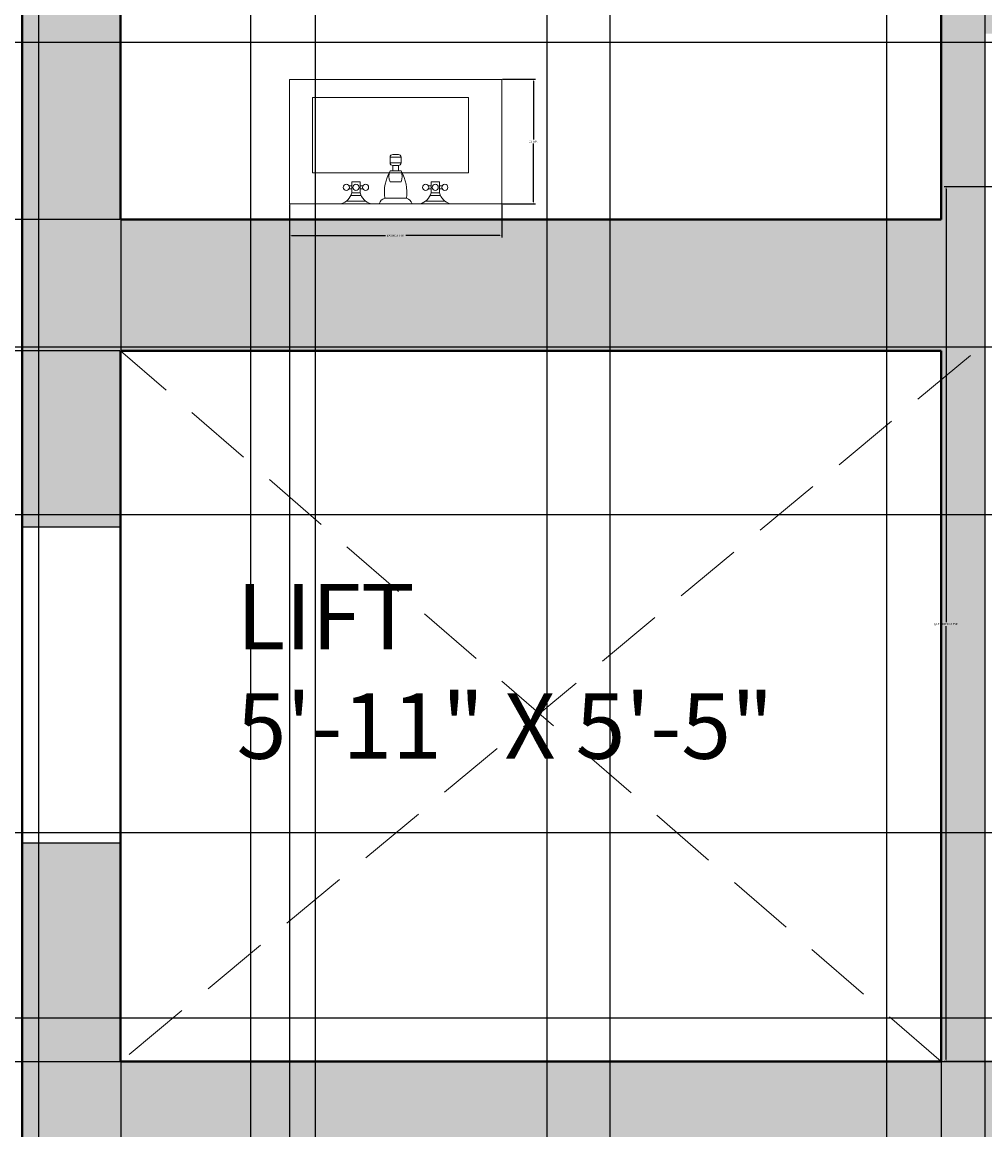
# Model space of a CAD drawing. Units: inches. Extents: x 818 to 1898, y 976 to 2364.
# Tile 50 of 96: x 1512 to 1600, y 1690 to 1791. Entities that reach past the tile are written whole.
import ezdxf

# ---------------------------------------------------------------- set-up
doc = ezdxf.new("R2010")
doc.units = ezdxf.units.IN
doc.header["$LTSCALE"] = 5
doc.header["$MEASUREMENT"] = 0
doc.linetypes.add('HIDDEN', pattern=[0.375, 0.25, -0.125])
for name, color, linetype, lineweight in [('A-ANNO-DIMS', 2, 'Continuous', 18), ('A-AREA-IDEN', 7, 'Continuous', 18), ('A-FLOR-FIXT', 9, 'Continuous', 18), ('A-FLOR-SHFT', 7, 'Continuous', 25), ('A-FLOR-SHFT-HIDN', 8, 'HIDDEN', 13), ('A-WALL', 7, 'Continuous', 40)]:
    doc.layers.add(name, color=color, linetype=linetype, lineweight=lineweight)
doc.layers.add('A-WALL-PATT', color=251, linetype='Continuous', lineweight=13, true_color=0x636466)
doc.styles.get("Standard").update_dxf_attribs({"font": 'arial.ttf'})
doc.dimstyles.get("Standard").update_dxf_attribs({"dimtxt": 0.18, "dimasz": 0.18, "dimexe": 0.18, "dimexo": 0.0625, "dimgap": 0.09, "dimtad": 0, "dimtih": 1, "dimtoh": 1, "dimdec": 4, "dimzin": 0, "dimdsep": 46, "dimtxsty": 'Standard', "dimcen": 0.09, "dimadec": 0, "dimazin": 0, "dimtfac": 1, "dimtdec": 4, "dimtofl": 0, "dimtmove": 0, "dimatfit": 3, "dimfxl": 1, "dimtolj": 1, "dimtzin": 0, "dimarcsym": 0})

# ---------------------------------------------------------------- blocks, each defined once
blk = doc.blocks.new('Faucet - Bathroom front')
for p, q in [((-0.5, 4.25), (0.5, 4.25)), ((0.5, 3.75), (-0.5, 3.75)), ((-0.25, 3), (-0.25, 3.5)), ((0.25, 3.5), (0.25, 3)), ((-0.5, 3), (0.5, 3)), ((-4, 1.625), (-4.25, 1.625)), ((-4, 1.375), (-4.25, 1.375)), ((-3.25, 1.625), (-3, 1.625)), ((-3.25, 1.375), (-3, 1.375)), ((0.5, 2), (-0.5, 2)), ((3.25, 1.625), (3, 1.625)), ((3.25, 1.375), (3, 1.375)), ((4, 1.625), (4.25, 1.625)), ((4, 1.375), (4.25, 1.375)), ((-5, 0), (-2.25, 0)), ((-4.5087, 0.25), (-2.7408, 0.25)), ((-3.1442, 0.75), (-4.0979, 0.75)), ((-1.5, 0), (1.5, 0)), ((-1, 0.5), (1, 0.5)), ((2.25, 0), (5, 0)), ((2.7413, 0.25), (4.5092, 0.25)), ((4.1058, 0.75), (3.1521, 0.75))]:
    blk.add_line(p, q)
for points in [[(-0.5, 3.75), (-0.5, 4.25)], [(-0.25, 4.5), (0.25, 4.5)], [(0.5, 4.25), (0.5, 3.75)], [(0.25, 3.5), (-0.25, 3.5)]]:
    blk.add_lwpolyline(points)
for points in [[(-4, 1), (-4, 2), (-3.25, 2), (-3.25, 1)], [(3.25, 1), (3.25, 2), (4, 2), (4, 1)]]:
    blk.add_lwpolyline(points, close=True)
for centre in [(-4.5, 1.5), (-3.625, 1.5), (-2.75, 1.5), (2.75, 1.5), (3.625, 1.5), (4.5, 1.5)]:
    blk.add_circle(centre, 0.2795)
for centre, radius, start, end in [((-0.2575, 4.2575), 0.2426, 88.22243, 181.7776), ((0.2575, 4.2575), 0.2426, 358.2224, 91.77757), ((-0.2575, 3.7425), 0.2426, 178.2224, 271.7776), ((0.2575, 3.7425), 0.2426, 268.2224, 1.777565), ((3, 1), 4.0311, 150.2551, 187.125), ((0.6413, 2.5), 1.246, 156.3417, 203.6583), ((-3, 1), 4.0311, 352.875, 29.74488), ((-0.6413, 2.5), 1.246, 336.3417, 23.65835), ((-5.375, 1.375), 1.4252, 285.2551, 344.7449), ((-1.875, 1.375), 1.4252, 195.2551, 254.7449), ((-0.7962, -0.2038), 0.7327, 106.1502, 163.8498), ((0.7962, -0.2038), 0.7327, 16.1502, 73.84979), ((1.875, 1.375), 1.4252, 285.2551, 344.7449), ((5.375, 1.375), 1.4252, 195.2551, 254.7449)]:
    blk.add_arc(centre, radius, start, end)
blk = doc.blocks.new('BASIN-COMPACT')
for points in [[(19.39, 0), (19.39, 11.38), (0, 11.38), (0, 0)], [(16.35, 2.84), (16.35, 9.72), (2.11, 9.72), (2.11, 2.84)]]:
    blk.add_lwpolyline(points, close=True)
blk = doc.blocks.new('*D46')
at = {"layer": 'A-ANNO-DIMS', "color": 0, "lineweight": -2, "ltscale": 5, "transparency": 16777216}
for p, q in [((1608.12, 1776.08), (1596, 1776.08)), ((1596.18, 1775.9), (1596.18, 1736.27)), ((1596.18, 1696.26), (1596.18, 1735.89)), ((1608.12, 1696.08), (1596, 1696.08))]:
    blk.add_line(p, q, dxfattribs=at)
at = {"layer": 'A-ANNO-DIMS', "color": 0, "ltscale": 5, "transparency": 16777216}
for points in [[(1596.15, 1775.9), (1596.21, 1775.9), (1596.18, 1776.08)], [(1596.15, 1696.26), (1596.21, 1696.26), (1596.18, 1696.08)]]:
    blk.add_solid(points, dxfattribs=at)
at = {"layer": 'Defpoints', "color": 0, "ltscale": 5, "transparency": 16777216}
for p in [(1608.18, 1776.08), (1596.18, 1696.08), (1608.18, 1696.08)]:
    blk.add_point(p, dxfattribs=at)
at = {"layer": 'A-ANNO-DIMS', "color": 0, "ltscale": 5, "transparency": 16777216, "insert": (1596.18, 1736.08), "char_height": 0.18, "attachment_point": 5}
blk.add_mtext('\\A1;QUEEN BED 80 TYP.', dxfattribs=at)
blk = doc.blocks.new('*D52')
at = {"layer": 'A-ANNO-DIMS', "color": 0, "lineweight": -2, "ltscale": 5, "transparency": 16777216}
for p, q in [((1536.17, 1774.47), (1536.17, 1771.44)), ((1555.56, 1774.47), (1555.56, 1771.44)), ((1536.35, 1771.62), (1544.93, 1771.62)), ((1555.38, 1771.62), (1546.8, 1771.62))]:
    blk.add_line(p, q, dxfattribs=at)
at = {"layer": 'A-ANNO-DIMS', "color": 0, "ltscale": 5, "transparency": 16777216}
for points in [[(1536.35, 1771.65), (1536.35, 1771.59), (1536.17, 1771.62)], [(1555.38, 1771.65), (1555.38, 1771.59), (1555.56, 1771.62)]]:
    blk.add_solid(points, dxfattribs=at)
at = {"layer": 'Defpoints', "color": 0, "ltscale": 5, "transparency": 16777216}
for p in [(1536.17, 1774.53), (1555.56, 1774.53), (1555.56, 1771.62)]:
    blk.add_point(p, dxfattribs=at)
at = {"layer": 'A-ANNO-DIMS', "color": 0, "ltscale": 5, "transparency": 16777216, "insert": (1545.86, 1771.62), "char_height": 0.18, "attachment_point": 5}
blk.add_mtext('\\A1;BASIN 19 TYP.', dxfattribs=at)
blk = doc.blocks.new('*D53')
at = {"layer": 'A-ANNO-DIMS', "color": 0, "lineweight": -2, "ltscale": 5, "transparency": 16777216}
for p, q in [((1555.62, 1785.91), (1558.64, 1785.91)), ((1558.46, 1785.73), (1558.46, 1780.4)), ((1558.46, 1774.71), (1558.46, 1780.04)), ((1555.62, 1774.53), (1558.64, 1774.53))]:
    blk.add_line(p, q, dxfattribs=at)
at = {"layer": 'A-ANNO-DIMS', "color": 0, "ltscale": 5, "transparency": 16777216}
for points in [[(1558.43, 1785.73), (1558.49, 1785.73), (1558.46, 1785.91)], [(1558.43, 1774.71), (1558.49, 1774.71), (1558.46, 1774.53)]]:
    blk.add_solid(points, dxfattribs=at)
at = {"layer": 'Defpoints', "color": 0, "ltscale": 5, "transparency": 16777216}
for p in [(1555.56, 1785.91), (1558.46, 1785.91), (1555.56, 1774.53)]:
    blk.add_point(p, dxfattribs=at)
at = {"layer": 'A-ANNO-DIMS', "color": 0, "ltscale": 5, "transparency": 16777216, "insert": (1558.46, 1780.22), "char_height": 0.18, "attachment_point": 5}
blk.add_mtext('\\A1;11 TYP.', dxfattribs=at)
blk = doc.blocks.new('*D85')
at = {"layer": 'A-ANNO-DIMS', "color": 0, "lineweight": -2, "ltscale": 5, "transparency": 16777216}
for p, q in [((1258.79, 2053.08), (1897.92, 2053.08)), ((1897.74, 2052.9), (1897.74, 1876.76)), ((1897.74, 1700.26), (1897.74, 1876.4)), ((1258.79, 1700.08), (1897.92, 1700.08))]:
    blk.add_line(p, q, dxfattribs=at)
at = {"layer": 'A-ANNO-DIMS', "color": 0, "ltscale": 5, "transparency": 16777216}
for points in [[(1897.71, 2052.9), (1897.77, 2052.9), (1897.74, 2053.08)], [(1897.71, 1700.26), (1897.77, 1700.26), (1897.74, 1700.08)]]:
    blk.add_solid(points, dxfattribs=at)
at = {"layer": 'Defpoints', "color": 0, "ltscale": 5, "transparency": 16777216}
for p in [(1258.73, 2053.08), (1897.74, 2053.08), (1258.73, 1700.08)]:
    blk.add_point(p, dxfattribs=at)
at = {"layer": 'A-ANNO-DIMS', "color": 0, "ltscale": 5, "transparency": 16777216, "insert": (1897.74, 1876.58), "char_height": 0.18, "attachment_point": 5}
blk.add_mtext('\\A1;353', dxfattribs=at)
blk = doc.blocks.new('*D101')
at = {"layer": 'A-ANNO-DIMS', "color": 0, "lineweight": -2, "ltscale": 5, "transparency": 16777216}
for p, q in [((1507.3, 1071.12), (1507.3, 2363.87)), ((1565.48, 1071.12), (1565.48, 2363.87)), ((1507.48, 2363.69), (1536, 2363.69)), ((1565.3, 2363.69), (1536.78, 2363.69))]:
    blk.add_line(p, q, dxfattribs=at)
at = {"layer": 'A-ANNO-DIMS', "color": 0, "ltscale": 5, "transparency": 16777216}
for points in [[(1507.48, 2363.72), (1507.48, 2363.66), (1507.3, 2363.69)], [(1565.3, 2363.72), (1565.3, 2363.66), (1565.48, 2363.69)]]:
    blk.add_solid(points, dxfattribs=at)
at = {"layer": 'Defpoints', "color": 0, "ltscale": 5, "transparency": 16777216}
for p in [(1565.48, 2363.69), (1507.3, 1071.06), (1565.48, 1071.06)]:
    blk.add_point(p, dxfattribs=at)
at = {"layer": 'A-ANNO-DIMS', "color": 0, "ltscale": 5, "transparency": 16777216, "insert": (1536.39, 2363.69), "char_height": 0.18, "attachment_point": 5}
blk.add_mtext('\\A1;58.19', dxfattribs=at)
blk = doc.blocks.new('*D102')
at = {"layer": 'A-ANNO-DIMS', "color": 0, "lineweight": -2, "ltscale": 5, "transparency": 16777216}
for p, q in [((1565.48, 1071.12), (1565.48, 2363.87)), ((1626.57, 1071.12), (1626.57, 2363.87)), ((1565.66, 2363.69), (1595.63, 2363.69)), ((1626.39, 2363.69), (1596.42, 2363.69))]:
    blk.add_line(p, q, dxfattribs=at)
at = {"layer": 'A-ANNO-DIMS', "color": 0, "ltscale": 5, "transparency": 16777216}
for points in [[(1565.66, 2363.72), (1565.66, 2363.66), (1565.48, 2363.69)], [(1626.39, 2363.72), (1626.39, 2363.66), (1626.57, 2363.69)]]:
    blk.add_solid(points, dxfattribs=at)
at = {"layer": 'Defpoints', "color": 0, "ltscale": 5, "transparency": 16777216}
for p in [(1626.57, 2363.69), (1565.48, 1071.06), (1626.57, 1071.06)]:
    blk.add_point(p, dxfattribs=at)
at = {"layer": 'A-ANNO-DIMS', "color": 0, "ltscale": 5, "transparency": 16777216, "insert": (1596.03, 2363.69), "char_height": 0.18, "attachment_point": 5}
blk.add_mtext('\\A1;61.09', dxfattribs=at)
blk = doc.blocks.new('*D119')
at = {"layer": 'A-ANNO-DIMS', "color": 0, "lineweight": -2, "ltscale": 5, "transparency": 16777216}
for p, q in [((1766.29, 1716.99), (818.03, 1716.99)), ((818.21, 1716.81), (818.21, 1672.43)), ((818.21, 1627.69), (818.21, 1672.06)), ((1766.29, 1627.51), (818.03, 1627.51))]:
    blk.add_line(p, q, dxfattribs=at)
at = {"layer": 'A-ANNO-DIMS', "color": 0, "ltscale": 5, "transparency": 16777216}
for points in [[(818.18, 1716.81), (818.24, 1716.81), (818.21, 1716.99)], [(818.18, 1627.69), (818.24, 1627.69), (818.21, 1627.51)]]:
    blk.add_solid(points, dxfattribs=at)
at = {"layer": 'Defpoints', "color": 0, "ltscale": 5, "transparency": 16777216}
for p in [(818.21, 1716.99), (1766.35, 1716.99), (1766.35, 1627.51)]:
    blk.add_point(p, dxfattribs=at)
at = {"layer": 'A-ANNO-DIMS', "color": 0, "ltscale": 5, "transparency": 16777216, "insert": (818.21, 1672.25), "char_height": 0.18, "attachment_point": 5}
blk.add_mtext('\\A1;89.48', dxfattribs=at)
blk = doc.blocks.new('*D120')
at = {"layer": 'A-ANNO-DIMS', "color": 0, "lineweight": -2, "ltscale": 5, "transparency": 16777216}
for p, q in [((1766.29, 1797.72), (818.03, 1797.72)), ((818.21, 1797.54), (818.21, 1757.53)), ((818.21, 1717.17), (818.21, 1757.17)), ((1766.29, 1716.99), (818.03, 1716.99))]:
    blk.add_line(p, q, dxfattribs=at)
at = {"layer": 'A-ANNO-DIMS', "color": 0, "ltscale": 5, "transparency": 16777216}
for points in [[(818.18, 1797.54), (818.24, 1797.54), (818.21, 1797.72)], [(818.18, 1717.17), (818.24, 1717.17), (818.21, 1716.99)]]:
    blk.add_solid(points, dxfattribs=at)
at = {"layer": 'Defpoints', "color": 0, "ltscale": 5, "transparency": 16777216}
for p in [(818.21, 1797.72), (1766.35, 1797.72), (1766.35, 1716.99)]:
    blk.add_point(p, dxfattribs=at)
at = {"layer": 'A-ANNO-DIMS', "color": 0, "ltscale": 5, "transparency": 16777216, "insert": (818.21, 1757.35), "char_height": 0.18, "attachment_point": 5}
blk.add_mtext('\\A1;80.73', dxfattribs=at)
blk = doc.blocks.new('*D175')
at = {"layer": 'A-ANNO-DIMS', "color": 0, "lineweight": -2, "ltscale": 5, "transparency": 16777216}
for p, q in [((1559.73, 1647.64), (1559.73, 2363.87)), ((1669.73, 1647.64), (1669.73, 2363.87)), ((1559.91, 2363.69), (1614.45, 2363.69)), ((1669.55, 2363.69), (1615.01, 2363.69))]:
    blk.add_line(p, q, dxfattribs=at)
at = {"layer": 'A-ANNO-DIMS', "color": 0, "ltscale": 5, "transparency": 16777216}
for points in [[(1559.91, 2363.72), (1559.91, 2363.66), (1559.73, 2363.69)], [(1669.55, 2363.72), (1669.55, 2363.66), (1669.73, 2363.69)]]:
    blk.add_solid(points, dxfattribs=at)
at = {"layer": 'Defpoints', "color": 0, "ltscale": 5, "transparency": 16777216}
for p in [(1669.73, 2363.69), (1559.73, 1647.58), (1669.73, 1647.58)]:
    blk.add_point(p, dxfattribs=at)
at = {"layer": 'A-ANNO-DIMS', "color": 0, "ltscale": 5, "transparency": 16777216, "insert": (1614.73, 2363.69), "char_height": 0.18, "attachment_point": 5}
blk.add_mtext('\\A1;110', dxfattribs=at)
blk = doc.blocks.new('*D215')
at = {"layer": 'A-ANNO-DIMS', "color": 0, "lineweight": -2, "ltscale": 5, "transparency": 16777216}
for p, q in [((1590.66, 1876.08), (818.03, 1876.08)), ((818.21, 1875.9), (818.21, 1781.76)), ((818.21, 1687.26), (818.21, 1781.4)), ((1511.66, 1687.08), (818.03, 1687.08))]:
    blk.add_line(p, q, dxfattribs=at)
at = {"layer": 'A-ANNO-DIMS', "color": 0, "ltscale": 5, "transparency": 16777216}
for points in [[(818.18, 1875.9), (818.24, 1875.9), (818.21, 1876.08)], [(818.18, 1687.26), (818.24, 1687.26), (818.21, 1687.08)]]:
    blk.add_solid(points, dxfattribs=at)
at = {"layer": 'Defpoints', "color": 0, "ltscale": 5, "transparency": 16777216}
for p in [(818.21, 1876.08), (1590.73, 1876.08), (1511.73, 1687.08)]:
    blk.add_point(p, dxfattribs=at)
at = {"layer": 'A-ANNO-DIMS', "color": 0, "ltscale": 5, "transparency": 16777216, "insert": (818.21, 1781.58), "char_height": 0.18, "attachment_point": 5}
blk.add_mtext('\\A1;189', dxfattribs=at)
blk = doc.blocks.new('*D219')
at = {"layer": 'A-ANNO-DIMS', "color": 0, "lineweight": -2, "ltscale": 5, "transparency": 16777216}
for p, q in [((1595.73, 1696.02), (1595.73, 975.66)), ((1599.73, 1696.02), (1599.73, 975.66)), ((1595.91, 975.84), (1597.57, 975.84)), ((1599.55, 975.84), (1597.88, 975.84))]:
    blk.add_line(p, q, dxfattribs=at)
at = {"layer": 'A-ANNO-DIMS', "color": 0, "ltscale": 5, "transparency": 16777216}
for points in [[(1595.91, 975.87), (1595.91, 975.81), (1595.73, 975.84)], [(1599.55, 975.87), (1599.55, 975.81), (1599.73, 975.84)]]:
    blk.add_solid(points, dxfattribs=at)
at = {"layer": 'Defpoints', "color": 0, "ltscale": 5, "transparency": 16777216}
for p in [(1595.73, 1696.08), (1599.73, 1696.08), (1599.73, 975.84)]:
    blk.add_point(p, dxfattribs=at)
at = {"layer": 'A-ANNO-DIMS', "color": 0, "ltscale": 5, "transparency": 16777216, "insert": (1597.73, 975.84), "char_height": 0.18, "attachment_point": 5}
blk.add_mtext('\\A1;4', dxfattribs=at)
blk = doc.blocks.new('*D220')
at = {"layer": 'A-ANNO-DIMS', "color": 0, "lineweight": -2, "ltscale": 5, "transparency": 16777216}
for p, q in [((1520.66, 1773.08), (818.03, 1773.08)), ((818.21, 1772.9), (818.21, 1767.26)), ((818.21, 1761.26), (818.21, 1766.9)), ((1520.66, 1761.08), (818.03, 1761.08))]:
    blk.add_line(p, q, dxfattribs=at)
at = {"layer": 'A-ANNO-DIMS', "color": 0, "ltscale": 5, "transparency": 16777216}
for points in [[(818.18, 1772.9), (818.24, 1772.9), (818.21, 1773.08)], [(818.18, 1761.26), (818.24, 1761.26), (818.21, 1761.08)]]:
    blk.add_solid(points, dxfattribs=at)
at = {"layer": 'Defpoints', "color": 0, "ltscale": 5, "transparency": 16777216}
for p in [(818.21, 1773.08), (1520.73, 1773.08), (1520.73, 1761.08)]:
    blk.add_point(p, dxfattribs=at)
at = {"layer": 'A-ANNO-DIMS', "color": 0, "ltscale": 5, "transparency": 16777216, "insert": (818.21, 1767.08), "char_height": 0.18, "attachment_point": 5}
blk.add_mtext('\\A1;12', dxfattribs=at)
blk = doc.blocks.new('*D224')
at = {"layer": 'A-ANNO-DIMS', "color": 0, "lineweight": -2, "ltscale": 5, "transparency": 16777216}
for p, q in [((1520.73, 1837.52), (1520.73, 975.66)), ((1532.59, 1837.52), (1532.59, 975.66)), ((1520.91, 975.84), (1526.2, 975.84)), ((1532.41, 975.84), (1527.11, 975.84))]:
    blk.add_line(p, q, dxfattribs=at)
at = {"layer": 'A-ANNO-DIMS', "color": 0, "ltscale": 5, "transparency": 16777216}
for points in [[(1520.91, 975.87), (1520.91, 975.81), (1520.73, 975.84)], [(1532.41, 975.87), (1532.41, 975.81), (1532.59, 975.84)]]:
    blk.add_solid(points, dxfattribs=at)
at = {"layer": 'Defpoints', "color": 0, "ltscale": 5, "transparency": 16777216}
for p in [(1520.73, 1837.58), (1532.59, 1837.58), (1532.59, 975.84)]:
    blk.add_point(p, dxfattribs=at)
at = {"layer": 'A-ANNO-DIMS', "color": 0, "ltscale": 5, "transparency": 16777216, "insert": (1526.66, 975.84), "char_height": 0.18, "attachment_point": 5}
blk.add_mtext('\\A1;11.868', dxfattribs=at)
blk = doc.blocks.new('*D226')
at = {"layer": 'A-ANNO-DIMS', "color": 0, "lineweight": -2, "ltscale": 5, "transparency": 16777216}
for p, q in [((1536.17, 1774.47), (1536.17, 975.66)), ((1520.73, 1773.02), (1520.73, 975.66)), ((1520.91, 975.84), (1527.99, 975.84)), ((1535.99, 975.84), (1528.9, 975.84))]:
    blk.add_line(p, q, dxfattribs=at)
at = {"layer": 'A-ANNO-DIMS', "color": 0, "ltscale": 5, "transparency": 16777216}
for points in [[(1520.91, 975.87), (1520.91, 975.81), (1520.73, 975.84)], [(1535.99, 975.87), (1535.99, 975.81), (1536.17, 975.84)]]:
    blk.add_solid(points, dxfattribs=at)
at = {"layer": 'Defpoints', "color": 0, "ltscale": 5, "transparency": 16777216}
for p in [(1536.17, 1774.53), (1520.73, 1773.08), (1536.17, 975.84)]:
    blk.add_point(p, dxfattribs=at)
at = {"layer": 'A-ANNO-DIMS', "color": 0, "ltscale": 5, "transparency": 16777216, "insert": (1528.45, 975.84), "char_height": 0.18, "attachment_point": 5}
blk.add_mtext('\\A1;15.445', dxfattribs=at)
blk = doc.blocks.new('*D229')
at = {"layer": 'A-ANNO-DIMS', "color": 0, "lineweight": -2, "ltscale": 5, "transparency": 16777216}
for p, q in [((1599.73, 2044.02), (1599.73, 975.66)), ((1620.14, 2036.06), (1620.14, 975.66)), ((1599.91, 975.84), (1609.47, 975.84)), ((1619.96, 975.84), (1610.4, 975.84))]:
    blk.add_line(p, q, dxfattribs=at)
at = {"layer": 'A-ANNO-DIMS', "color": 0, "ltscale": 5, "transparency": 16777216}
for points in [[(1599.91, 975.87), (1599.91, 975.81), (1599.73, 975.84)], [(1619.96, 975.87), (1619.96, 975.81), (1620.14, 975.84)]]:
    blk.add_solid(points, dxfattribs=at)
at = {"layer": 'Defpoints', "color": 0, "ltscale": 5, "transparency": 16777216}
for p in [(1599.73, 2044.08), (1620.14, 2036.12), (1620.14, 975.84)]:
    blk.add_point(p, dxfattribs=at)
at = {"layer": 'A-ANNO-DIMS', "color": 0, "ltscale": 5, "transparency": 16777216, "insert": (1609.93, 975.84), "char_height": 0.18, "attachment_point": 5}
blk.add_mtext('\\A1;20.416', dxfattribs=at)
blk = doc.blocks.new('*D242')
at = {"layer": 'A-ANNO-DIMS', "color": 0, "lineweight": -2, "ltscale": 5, "transparency": 16777216}
for p, q in [((1488.26, 1948.6), (1488.26, 975.66)), ((1513.23, 1948.6), (1513.23, 975.66)), ((1488.44, 975.84), (1500.35, 975.84)), ((1513.05, 975.84), (1501.14, 975.84))]:
    blk.add_line(p, q, dxfattribs=at)
at = {"layer": 'A-ANNO-DIMS', "color": 0, "ltscale": 5, "transparency": 16777216}
for points in [[(1488.44, 975.87), (1488.44, 975.81), (1488.26, 975.84)], [(1513.05, 975.87), (1513.05, 975.81), (1513.23, 975.84)]]:
    blk.add_solid(points, dxfattribs=at)
at = {"layer": 'Defpoints', "color": 0, "ltscale": 5, "transparency": 16777216}
for p in [(1488.26, 1948.66), (1513.23, 1948.66), (1513.23, 975.84)]:
    blk.add_point(p, dxfattribs=at)
at = {"layer": 'A-ANNO-DIMS', "color": 0, "ltscale": 5, "transparency": 16777216, "insert": (1500.74, 975.84), "char_height": 0.18, "attachment_point": 5}
blk.add_mtext('\\A1;24.97', dxfattribs=at)
blk = doc.blocks.new('*D243')
at = {"layer": 'A-ANNO-DIMS', "color": 0, "lineweight": -2, "ltscale": 5, "transparency": 16777216}
for p, q in [((1451.77, 2020.02), (1451.77, 975.66)), ((1590.73, 2020.02), (1590.73, 975.66)), ((1451.95, 975.84), (1520.79, 975.84)), ((1590.55, 975.84), (1521.7, 975.84))]:
    blk.add_line(p, q, dxfattribs=at)
at = {"layer": 'A-ANNO-DIMS', "color": 0, "ltscale": 5, "transparency": 16777216}
for points in [[(1451.95, 975.87), (1451.95, 975.81), (1451.77, 975.84)], [(1590.55, 975.87), (1590.55, 975.81), (1590.73, 975.84)]]:
    blk.add_solid(points, dxfattribs=at)
at = {"layer": 'Defpoints', "color": 0, "ltscale": 5, "transparency": 16777216}
for p in [(1451.77, 2020.08), (1590.73, 2020.08), (1590.73, 975.84)]:
    blk.add_point(p, dxfattribs=at)
at = {"layer": 'A-ANNO-DIMS', "color": 0, "ltscale": 5, "transparency": 16777216, "insert": (1521.25, 975.84), "char_height": 0.18, "attachment_point": 5}
blk.add_mtext('\\A1;138.96', dxfattribs=at)
blk = doc.blocks.new('*D253')
at = {"layer": 'A-ANNO-DIMS', "color": 0, "lineweight": -2, "ltscale": 5, "transparency": 16777216}
for p, q in [((1485.12, 2053.02), (1485.12, 975.66)), ((1538.52, 2053.02), (1538.52, 975.66)), ((1485.3, 975.84), (1511.42, 975.84)), ((1538.34, 975.84), (1512.21, 975.84))]:
    blk.add_line(p, q, dxfattribs=at)
at = {"layer": 'A-ANNO-DIMS', "color": 0, "ltscale": 5, "transparency": 16777216}
for points in [[(1485.3, 975.87), (1485.3, 975.81), (1485.12, 975.84)], [(1538.34, 975.87), (1538.34, 975.81), (1538.52, 975.84)]]:
    blk.add_solid(points, dxfattribs=at)
at = {"layer": 'Defpoints', "color": 0, "ltscale": 5, "transparency": 16777216}
for p in [(1485.12, 2053.08), (1538.52, 2053.08), (1538.52, 975.84)]:
    blk.add_point(p, dxfattribs=at)
at = {"layer": 'A-ANNO-DIMS', "color": 0, "ltscale": 5, "transparency": 16777216, "insert": (1511.82, 975.84), "char_height": 0.18, "attachment_point": 5}
blk.add_mtext('\\A1;53.39', dxfattribs=at)
blk = doc.blocks.new('*D280')
at = {"layer": 'A-ANNO-DIMS', "color": 0, "lineweight": -2, "ltscale": 5, "transparency": 16777216}
for p, q in [((1398.73, 1789.31), (1897.92, 1789.31)), ((1897.74, 1789.13), (1897.74, 1767.89)), ((1897.74, 1746.29), (1897.74, 1767.53)), ((1397.41, 1746.11), (1897.92, 1746.11))]:
    blk.add_line(p, q, dxfattribs=at)
at = {"layer": 'A-ANNO-DIMS', "color": 0, "ltscale": 5, "transparency": 16777216}
for points in [[(1897.71, 1789.13), (1897.77, 1789.13), (1897.74, 1789.31)], [(1897.71, 1746.29), (1897.77, 1746.29), (1897.74, 1746.11)]]:
    blk.add_solid(points, dxfattribs=at)
at = {"layer": 'Defpoints', "color": 0, "ltscale": 5, "transparency": 16777216}
for p in [(1398.67, 1789.31), (1897.74, 1789.31), (1397.35, 1746.11)]:
    blk.add_point(p, dxfattribs=at)
at = {"layer": 'A-ANNO-DIMS', "color": 0, "ltscale": 5, "transparency": 16777216, "insert": (1897.74, 1767.71), "char_height": 0.18, "attachment_point": 5}
blk.add_mtext('\\A1;43.19', dxfattribs=at)
blk = doc.blocks.new('*D282')
at = {"layer": 'A-ANNO-DIMS', "color": 0, "lineweight": -2, "ltscale": 5, "transparency": 16777216}
for p, q in [((1422.08, 2081.19), (1897.92, 2081.19)), ((1897.74, 2081.01), (1897.74, 1884.32)), ((1897.74, 1687.26), (1897.74, 1883.95)), ((1463.79, 1687.08), (1897.92, 1687.08))]:
    blk.add_line(p, q, dxfattribs=at)
at = {"layer": 'A-ANNO-DIMS', "color": 0, "ltscale": 5, "transparency": 16777216}
for points in [[(1897.71, 2081.01), (1897.77, 2081.01), (1897.74, 2081.19)], [(1897.71, 1687.26), (1897.77, 1687.26), (1897.74, 1687.08)]]:
    blk.add_solid(points, dxfattribs=at)
at = {"layer": 'Defpoints', "color": 0, "ltscale": 5, "transparency": 16777216}
for p in [(1422.02, 2081.19), (1897.74, 2081.19), (1463.73, 1687.08)]:
    blk.add_point(p, dxfattribs=at)
at = {"layer": 'A-ANNO-DIMS', "color": 0, "ltscale": 5, "transparency": 16777216, "insert": (1897.74, 1884.13), "char_height": 0.18, "attachment_point": 5}
blk.add_mtext('\\A1;394.1', dxfattribs=at)
blk = doc.blocks.new('*D284')
at = {"layer": 'A-ANNO-DIMS', "color": 0, "lineweight": -2, "ltscale": 5, "transparency": 16777216}
for p, q in [((1351.66, 1761.45), (1897.92, 1761.45)), ((1897.74, 1761.27), (1897.74, 1728.95)), ((1897.74, 1696.26), (1897.74, 1728.58)), ((1267.79, 1696.08), (1897.92, 1696.08))]:
    blk.add_line(p, q, dxfattribs=at)
at = {"layer": 'A-ANNO-DIMS', "color": 0, "ltscale": 5, "transparency": 16777216}
for points in [[(1897.71, 1761.27), (1897.77, 1761.27), (1897.74, 1761.45)], [(1897.71, 1696.26), (1897.77, 1696.26), (1897.74, 1696.08)]]:
    blk.add_solid(points, dxfattribs=at)
at = {"layer": 'Defpoints', "color": 0, "ltscale": 5, "transparency": 16777216}
for p in [(1351.6, 1761.45), (1267.73, 1696.08), (1897.74, 1696.08)]:
    blk.add_point(p, dxfattribs=at)
at = {"layer": 'A-ANNO-DIMS', "color": 0, "ltscale": 5, "transparency": 16777216, "insert": (1897.74, 1728.76), "char_height": 0.18, "attachment_point": 5}
blk.add_mtext('\\A1;65.37', dxfattribs=at)

msp = doc.modelspace()

# ---------------------------------------------------------------- hatches: boundary and pattern name
at = {"layer": 'A-WALL-PATT', "ltscale": 5}
h = msp.add_hatch(color=256, dxfattribs=at)
h.dxf.hatch_style = 1
h.paths.add_polyline_path([(1267.7251, 1928.9218), (1258.7251, 1928.9218), (1258.7251, 1913.6401), (1250.3029, 1913.6401), (1250.3029, 1878.3919), (1258.7251, 1878.3919), (1258.7251, 1862.9652), (1267.7251, 1862.9652)])
h.paths.add_polyline_path([(1267.7251, 1814.9652), (1258.7251, 1814.9652), (1258.7251, 1755.3321), (1267.7251, 1755.3321)])
h.paths.add_polyline_path([(1463.7251, 1696.0782), (1267.7251, 1696.0782), (1267.7251, 1707.3321), (1258.7251, 1707.3321), (1258.7251, 1700.0782), (1251.9333, 1700.0782), (1251.9333, 1687.0782), (1463.7251, 1687.0782)])
h.paths.add_polyline_path([(1714.7252, 1717.3178), (1705.7252, 1717.3178), (1705.7252, 1696.0782), (1599.7251, 1696.0782), (1599.7251, 1790.0782), (1705.7252, 1790.0782), (1705.7252, 1785.6125), (1714.7252, 1785.6125), (1714.7252, 1827.2125), (1705.7252, 1827.2125), (1705.7252, 1802.0782), (1599.7251, 1802.0782), (1599.7251, 1867.0782), (1705.7252, 1867.0782), (1705.7252, 1857.2125), (1714.7252, 1857.2125), (1714.7252, 1930.0316), (1741.8409, 1930.0316), (1741.8409, 1935.0316), (1714.7252, 1935.0316), (1714.7252, 1957.0338), (1741.8409, 1957.0338), (1741.8409, 1962.0338), (1714.7252, 1962.0338), (1705.7252, 1962.0338), (1705.7252, 1948.0782), (1599.7251, 1948.0782), (1599.7251, 1981.0782), (1590.7251, 1981.0782), (1590.7251, 1941.0782), (1620.7252, 1941.0782), (1705.7252, 1941.0782), (1705.7252, 1876.0782), (1599.7251, 1876.0782), (1599.7251, 1911.0782), (1590.7251, 1911.0782), (1590.7251, 1876.0782), (1429.2252, 1876.0782), (1429.2252, 1867.0782), (1511.7251, 1867.0782), (1528.593, 1867.0782), (1595.7251, 1867.0782), (1595.7251, 1773.0782), (1520.7251, 1773.0782), (1520.7251, 1837.5823), (1532.593, 1837.5823), (1532.593, 1867.0782), (1528.593, 1867.0782), (1528.593, 1841.5823), (1511.7251, 1841.5823), (1511.7251, 1744.9714), (1520.7251, 1744.9714), (1520.7251, 1761.0782), (1595.7251, 1761.0782), (1595.7251, 1696.0782), (1520.7251, 1696.0782), (1520.7251, 1716.0454), (1511.7251, 1716.0454), (1511.7251, 1696.0782), (1511.7251, 1687.0782), (1714.7252, 1687.0782)])
h.paths.add_polyline_path([(1714.7252, 2053.0782), (1714.7252, 2081.1881), (1709.7252, 2081.1881), (1709.7252, 2053.0782), (1681.6446, 2053.0782), (1681.6446, 2081.1881), (1676.6446, 2081.1881), (1676.6446, 2053.0782), (1538.5155, 2053.0782), (1538.5155, 2044.0782), (1590.7251, 2044.0782), (1590.7251, 2011.0782), (1599.7251, 2011.0782), (1599.7251, 2044.0782), (1705.7252, 2044.0782), (1705.7252, 2014.5114), (1714.7252, 2014.5114)])
h.paths.add_polyline_path([(1485.1216, 2053.0782), (1422.02, 2053.0782), (1422.02, 2081.1881), (1413.02, 2081.1881), (1413.02, 2053.0782), (1399.6356, 2053.0782), (1399.6356, 2081.1881), (1390.6356, 2081.1881), (1390.6356, 2053.0782), (1388.0315, 2053.0782), (1388.0315, 2044.0782), (1416.2743, 2044.0782), (1485.1216, 2044.0782)])
h.paths.add_polyline_path([(1330.305, 2053.0782), (1258.7251, 2053.0782), (1258.7251, 2019.2871), (1267.7251, 2019.2871), (1267.7251, 2044.0782), (1330.305, 2044.0782)])
h.paths.add_polyline_path([(1258.7251, 2053.0782), (1214.6577, 2053.0782), (1214.6577, 2044.0782), (1258.7251, 2044.0782)])
h.paths.add_polyline_path([(1214.6577, 2053.0782), (1180.349, 2053.0782), (1180.349, 2044.0782), (1214.6577, 2044.0782)])
h.paths.add_polyline_path([(1714.7252, 1639.5782), (1741.8409, 1639.5782), (1741.8409, 1643.5782), (1714.7252, 1643.5782), (1714.7252, 1649.9029), (1705.7252, 1649.9029), (1705.7252, 1600.0782), (1477.7252, 1600.0782), (1477.7252, 1591.0782), (1520.7251, 1591.0782), (1616.7252, 1591.0782), (1616.7252, 1416.6857), (1622.7252, 1416.6857), (1622.7252, 1463.0782), (1624.7252, 1463.0782), (1624.7252, 1467.0782), (1622.7252, 1467.0782), (1622.7252, 1591.0782), (1705.7252, 1591.0782), (1705.7252, 1545.0782), (1714.7252, 1545.0782), (1741.8409, 1545.0782), (1741.8409, 1549.0782), (1714.7252, 1549.0782), (1714.7252, 1593.9175), (1737.8409, 1593.9175), (1737.8409, 1597.9175), (1714.7252, 1597.9175)])
h.paths.add_polyline_path([(1674.9024, 2060.7419), (1714.7045, 2060.7419), (1714.7045, 2073.1061), (1674.9024, 2073.1061)], flags=25)
h.paths.add_polyline_path([(1394.5468, 2061.6618), (1422.2344, 2061.6618), (1422.2344, 2074.0261), (1394.5468, 2074.0261)], flags=24)

# ---------------------------------------------------------------- linework, layer by layer
at = {"layer": 'A-FLOR-SHFT'}
msp.add_lwpolyline([(1511.7251, 1744.9714), (1520.7251, 1744.9714), (1520.7251, 1716.0454), (1511.7251, 1716.0454)], close=True, dxfattribs=at)
at = {"layer": 'A-FLOR-SHFT-HIDN', "ltscale": 5}
for p, q in [((1595.7251, 1696.0782), (1520.7251, 1761.0782)), ((1598.4151, 1760.6396), (1520.7251, 1696.0782))]:
    msp.add_line(p, q, dxfattribs=at)
at = {"layer": 'A-WALL'}
for p, q in [((1595.7251, 1867.0782), (1595.7251, 1773.0782)), ((1511.7251, 1841.5823), (1511.7251, 1696.0782)), ((1520.7251, 1837.5823), (1520.7251, 1773.0782)), ((1520.7251, 1773.0782), (1595.7251, 1773.0782)), ((1520.7251, 1761.0782), (1595.7251, 1761.0782)), ((1520.7251, 1761.0782), (1520.7251, 1696.0782)), ((1595.7251, 1761.0782), (1595.7251, 1696.0782)), ((1511.7251, 1696.0782), (1511.7251, 1687.0782)), ((1520.7251, 1696.0782), (1595.7251, 1696.0782))]:
    msp.add_line(p, q, dxfattribs=at)

# ---------------------------------------------------------------- block references
at = {"layer": 'A-FLOR-FIXT'}
for name, p in [('BASIN-COMPACT', (1536.17, 1774.528)), ('Faucet - Bathroom front', (1545.863, 1774.5283))]:
    msp.add_blockref(name, p, dxfattribs=at)

# ---------------------------------------------------------------- texts
at = {"layer": 'A-AREA-IDEN', "ltscale": 5, "insert": (1531.3401, 1739.7621), "char_height": 6, "attachment_point": 1}
msp.add_mtext_dynamic_manual_height_columns('LIFT\\P5\'-11" X 5\'-5"', width=118.992422, gutter_width=1, heights=[0], dxfattribs=at)

# ---------------------------------------------------------------- dimensions: what is measured, and where the dimension line sits
at = {"layer": 'A-ANNO-DIMS', "ltscale": 5}
for base, p1, p2, override, picture, middle in [((1565.4835, 2363.6929), (1507.2982, 1071.0552), (1565.4835, 1071.0552), {"dimdec": 2, "dimlfac": 1, "dimrnd": 0, "dimzin": 0, "dimdsep": 46, "dimlunit": 2}, '*D101', (1536.3908, 2363.6929)), ((1669.7251, 2363.6929), (1559.7251, 1647.5782), (1669.7251, 1647.5782), {"dimdec": 0, "dimlfac": 1, "dimrnd": 0, "dimzin": 0, "dimdsep": 46, "dimlunit": 2}, '*D175', (1614.7251, 2363.6929)), ((1626.5748, 2363.6929), (1565.4835, 1071.0552), (1626.5748, 1071.0552), {"dimdec": 2, "dimlfac": 1, "dimrnd": 0, "dimzin": 0, "dimdsep": 46, "dimlunit": 2}, '*D102', (1596.0291, 2363.6929)), ((1538.5155, 975.8433), (1485.1216, 2053.0782), (1538.5155, 2053.0782), {"dimdec": 2, "dimlfac": 1, "dimrnd": 0, "dimzin": 0, "dimdsep": 46, "dimlunit": 2}, '*D253', (1511.8185, 975.8433)), ((1620.14159, 975.84326), (1599.72515, 2044.07824), (1620.14159, 2036.1182), {"dimdec": 3, "dimlfac": 1, "dimrnd": 0, "dimzin": 0, "dimdsep": 46, "dimlunit": 2}, '*D229', (1609.93337, 975.84326)), ((1590.7251, 975.8433), (1451.7698, 2020.0782), (1590.7251, 2020.0782), {"dimdec": 2, "dimlfac": 1, "dimrnd": 0, "dimzin": 0, "dimdsep": 46, "dimlunit": 2}, '*D243', (1521.2475, 975.8433)), ((1513.2306, 975.8433), (1488.2586, 1948.6602), (1513.2306, 1948.6602), {"dimdec": 2, "dimlfac": 1, "dimrnd": 0, "dimzin": 0, "dimdsep": 46, "dimlunit": 2}, '*D242', (1500.7446, 975.8433)), ((1532.593, 975.8433), (1520.7251, 1837.5823), (1532.593, 1837.5823), {"dimdec": 3, "dimlfac": 1, "dimrnd": 0, "dimzin": 0, "dimdsep": 46, "dimlunit": 2}, '*D224', (1526.6591, 975.8433)), ((1536.1698, 975.8433), (1520.7251, 1773.0782), (1536.1698, 1774.5283), {"dimdec": 3, "dimlfac": 1, "dimrnd": 0, "dimzin": 0, "dimdsep": 46, "dimlunit": 2}, '*D226', (1528.4475, 975.8433)), ((1599.7251, 975.8433), (1595.7251, 1696.0782), (1599.7251, 1696.0782), {"dimdec": 0, "dimlfac": 1, "dimrnd": 0, "dimzin": 0, "dimdsep": 46, "dimlunit": 2}, '*D219', (1597.7251, 975.8433))]:
    dim = msp.add_linear_dim(base=base, p1=p1, p2=p2, dimstyle='Standard', override=override, dxfattribs=at)
    dim.commit()
    dim.dimension.update_dxf_attribs({"geometry": picture, "text_midpoint": middle})
for base, p1, p2, override, picture, middle in [((1897.736, 2081.1881), (1463.7251, 1687.0782), (1422.02, 2081.1881), {"dimdec": 1, "dimlfac": 1, "dimrnd": 0, "dimzin": 0, "dimdsep": 46, "dimlunit": 2}, '*D282', (1897.736, 1884.1332)), ((1897.736, 2053.0782), (1258.7251, 1700.0782), (1258.7251, 2053.0782), {"dimdec": 0, "dimlfac": 1, "dimrnd": 0, "dimzin": 0, "dimdsep": 46, "dimlunit": 2}, '*D85', (1897.736, 1876.5782)), ((818.2059, 1876.0782), (1511.7251, 1687.0782), (1590.7251, 1876.0782), {"dimdec": 0, "dimlfac": 1, "dimrnd": 0, "dimzin": 0, "dimdsep": 46, "dimlunit": 2}, '*D215', (818.2059, 1781.5782)), ((818.2059, 1797.7165), (1766.3524, 1716.9866), (1766.3524, 1797.7165), {"dimdec": 2, "dimlfac": 1, "dimrnd": 0, "dimzin": 0, "dimdsep": 46, "dimlunit": 2}, '*D120', (818.2059, 1757.3516)), ((1897.736, 1789.3057), (1397.3459, 1746.1142), (1398.6717, 1789.3057), {"dimdec": 2, "dimlfac": 1, "dimrnd": 0, "dimzin": 0, "dimdsep": 46, "dimlunit": 2}, '*D280', (1897.736, 1767.71)), ((818.2059, 1773.0782), (1520.7251, 1761.0782), (1520.7251, 1773.0782), {"dimdec": 0, "dimlfac": 1, "dimrnd": 0, "dimzin": 0, "dimdsep": 46, "dimlunit": 2}, '*D220', (818.2059, 1767.0782)), ((1897.736, 1696.0782), (1351.5985, 1761.449), (1267.7251, 1696.0782), {"dimdec": 2, "dimlfac": 1, "dimrnd": 0, "dimzin": 0, "dimdsep": 46, "dimlunit": 2}, '*D284', (1897.736, 1728.7636)), ((818.2059, 1716.9866), (1766.3524, 1627.5052), (1766.3524, 1716.9866), {"dimdec": 2, "dimlfac": 1, "dimrnd": 0, "dimzin": 0, "dimdsep": 46, "dimlunit": 2}, '*D119', (818.2059, 1672.2459))]:
    dim = msp.add_linear_dim(base=base, p1=p1, p2=p2, angle=90, dimstyle='Standard', override=override, dxfattribs=at)
    dim.commit()
    dim.dimension.update_dxf_attribs({"geometry": picture, "text_midpoint": middle})
for base, p1, p2, angle, text, picture, middle in [((1558.4641, 1785.9107), (1555.5561, 1774.5283), (1555.5561, 1785.9107), 90, '<> TYP.', '*D53', (1558.4641, 1780.2195)), ((1596.1841, 1696.0782), (1608.1842, 1776.0783), (1608.1842, 1696.0782), 270, 'QUEEN BED <> TYP.', '*D46', (1596.1841, 1736.0783))]:
    dim = msp.add_linear_dim(base=base, p1=p1, p2=p2, angle=angle, text=text, dimstyle='Standard', override={"dimdec": 0, "dimlfac": 1, "dimrnd": 0, "dimzin": 0, "dimdsep": 46, "dimlunit": 2}, dxfattribs=at)
    dim.commit()
    dim.dimension.update_dxf_attribs({"geometry": picture, "text_midpoint": middle})
dim = msp.add_linear_dim(base=(1555.5561, 1771.6204), p1=(1536.1698, 1774.5283), p2=(1555.5561, 1774.5283), text='BASIN <> TYP.', dimstyle='Standard', override={"dimdec": 0, "dimlfac": 1, "dimrnd": 0, "dimzin": 0, "dimdsep": 46, "dimlunit": 2}, dxfattribs=at)
dim.commit()
dim.dimension.update_dxf_attribs({"geometry": '*D52', "text_midpoint": (1545.863, 1771.6204)})

doc.saveas('drawing.dxf')
